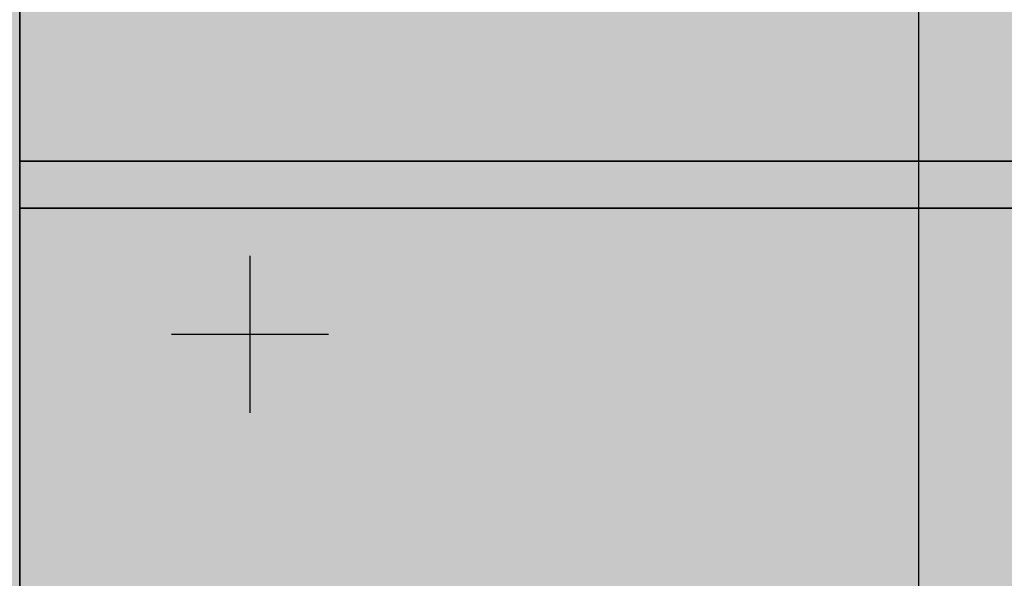
# Model space of a CAD drawing. Units: millimetres. Extents: x 130 to 1021, y 147 to 699.
# Tile 31 of 40: x 487 to 550, y 440 to 476. Entities that reach past the tile are written whole.
import ezdxf

# ---------------------------------------------------------------- set-up
doc = ezdxf.new("R2010")
doc.units = ezdxf.units.MM
doc.header["$MEASUREMENT"] = 0
for name, color, linetype, lineweight in [('A-ANNO-DIMS', 2, 'Continuous', 18), ('A-ELEV', 7, 'Continuous', 35), ('A-ELEV-PATT', 9, 'Continuous', 13)]:
    doc.layers.add(name, color=color, linetype=linetype, lineweight=lineweight)
doc.styles.get("Standard").update_dxf_attribs({"font": 'arial.ttf'})
doc.dimstyles.get("Standard").update_dxf_attribs({"dimtxt": 20, "dimasz": 10, "dimexe": 10, "dimexo": 10, "dimgap": 5, "dimtad": 0, "dimtih": 1, "dimtoh": 1, "dimdec": 0, "dimzin": 0, "dimdsep": 46, "dimtxsty": 'Standard', "dimcen": 5, "dimadec": 0, "dimazin": 0, "dimtfac": 1, "dimtdec": 0, "dimtofl": 0, "dimtmove": 0, "dimatfit": 3, "dimfxl": 1, "dimtolj": 1, "dimtzin": 0, "dimarcsym": 0})

# ---------------------------------------------------------------- blocks, each defined once
blk = doc.blocks.new('*D11')
at = {"layer": 'A-ANNO-DIMS', "color": 0, "lineweight": -2, "transparency": 16777216}
for p, q in [((737.374, 648.699), (737.374, 149.739)), ((299.374, 566.947), (299.374, 149.739)), ((309.374, 159.739), (490.857, 159.739)), ((727.374, 159.739), (545.891, 159.739))]:
    blk.add_line(p, q, dxfattribs=at)
at = {"layer": 'A-ANNO-DIMS', "color": 0, "transparency": 16777216}
for points in [[(309.374, 161.406), (309.374, 158.073), (299.374, 159.739)], [(727.374, 161.406), (727.374, 158.073), (737.374, 159.739)]]:
    blk.add_solid(points, dxfattribs=at)
at = {"layer": 'Defpoints', "color": 0, "transparency": 16777216}
for p in [(737.374, 658.699), (299.374, 576.947), (737.374, 159.739)]:
    blk.add_point(p, dxfattribs=at)
at = {"layer": 'A-ANNO-DIMS', "color": 0, "transparency": 16777216, "insert": (518.374, 159.739), "char_height": 20, "attachment_point": 5}
blk.add_mtext('\\A1;438', dxfattribs=at)
blk = doc.blocks.new('*D12')
at = {"layer": 'A-ANNO-DIMS', "color": 0, "lineweight": -2, "transparency": 16777216}
for p, q in [((477.374, 661.947), (265.074, 661.947)), ((275.074, 651.947), (275.074, 438.205)), ((275.074, 194.039), (275.074, 407.782)), ((357.163, 184.039), (265.074, 184.039))]:
    blk.add_line(p, q, dxfattribs=at)
at = {"layer": 'A-ANNO-DIMS', "color": 0, "transparency": 16777216}
for points in [[(273.407, 651.947), (276.74, 651.947), (275.074, 661.947)], [(273.407, 194.039), (276.74, 194.039), (275.074, 184.039)]]:
    blk.add_solid(points, dxfattribs=at)
at = {"layer": 'Defpoints', "color": 0, "transparency": 16777216}
for p in [(275.074, 661.947), (487.374, 661.947), (367.163, 184.039)]:
    blk.add_point(p, dxfattribs=at)
at = {"layer": 'A-ANNO-DIMS', "color": 0, "transparency": 16777216, "insert": (275.074, 422.993), "char_height": 20, "attachment_point": 5}
blk.add_mtext('\\A1;477.9', dxfattribs=at)
blk = doc.blocks.new('*D19')
at = {"layer": 'A-ANNO-DIMS', "color": 0, "lineweight": -2, "transparency": 16777216}
for p, q in [((382.374, 388.947), (382.374, 696.247)), ((414.652, 510.881), (414.652, 696.247)), ((392.374, 686.247), (404.652, 686.247)), ((414.652, 686.247), (424.652, 686.247))]:
    blk.add_line(p, q, dxfattribs=at)
at = {"layer": 'A-ANNO-DIMS', "color": 0, "transparency": 16777216}
for points in [[(392.374, 687.914), (392.374, 684.581), (382.374, 686.247)], [(404.652, 687.914), (404.652, 684.581), (414.652, 686.247)]]:
    blk.add_solid(points, dxfattribs=at)
at = {"layer": 'Defpoints', "color": 0, "transparency": 16777216}
for p in [(414.652, 686.247), (414.652, 500.881), (382.374, 378.947)]:
    blk.add_point(p, dxfattribs=at)
at = {"layer": 'A-ANNO-DIMS', "color": 0, "transparency": 16777216, "insert": (463.411, 686.247), "char_height": 20, "attachment_point": 5}
blk.add_mtext('\\A1;32.28', dxfattribs=at)
blk = doc.blocks.new('*D20')
at = {"layer": 'A-ANNO-DIMS', "color": 0, "lineweight": -2, "transparency": 16777216}
for p, q in [((414.652, 510.881), (414.652, 696.247)), ((432.374, 388.947), (432.374, 696.247)), ((404.652, 686.247), (394.652, 686.247)), ((442.374, 686.247), (452.374, 686.247))]:
    blk.add_line(p, q, dxfattribs=at)
at = {"layer": 'A-ANNO-DIMS', "color": 0, "transparency": 16777216}
for points in [[(404.652, 687.914), (404.652, 684.581), (414.652, 686.247)], [(442.374, 687.914), (442.374, 684.581), (432.374, 686.247)]]:
    blk.add_solid(points, dxfattribs=at)
at = {"layer": 'Defpoints', "color": 0, "transparency": 16777216}
for p in [(432.374, 686.247), (414.652, 500.881), (432.374, 378.947)]:
    blk.add_point(p, dxfattribs=at)
at = {"layer": 'A-ANNO-DIMS', "color": 0, "transparency": 16777216, "insert": (490.075, 686.247), "char_height": 20, "attachment_point": 5}
blk.add_mtext('\\A1;17.72', dxfattribs=at)
blk = doc.blocks.new('*D21')
at = {"layer": 'A-ANNO-DIMS', "color": 0, "lineweight": -2, "transparency": 16777216}
for p, q in [((432.374, 388.947), (432.374, 696.247)), ((447.374, 656.947), (447.374, 696.247)), ((422.374, 686.247), (412.374, 686.247)), ((457.374, 686.247), (467.374, 686.247))]:
    blk.add_line(p, q, dxfattribs=at)
at = {"layer": 'A-ANNO-DIMS', "color": 0, "transparency": 16777216}
for points in [[(422.374, 687.914), (422.374, 684.581), (432.374, 686.247)], [(457.374, 687.914), (457.374, 684.581), (447.374, 686.247)]]:
    blk.add_solid(points, dxfattribs=at)
at = {"layer": 'Defpoints', "color": 0, "transparency": 16777216}
for p in [(447.374, 686.247), (447.374, 646.947), (432.374, 378.947)]:
    blk.add_point(p, dxfattribs=at)
at = {"layer": 'A-ANNO-DIMS', "color": 0, "transparency": 16777216, "insert": (485.832, 686.247), "char_height": 20, "attachment_point": 5}
blk.add_mtext('\\A1;15', dxfattribs=at)
blk = doc.blocks.new('*D22')
at = {"layer": 'A-ANNO-DIMS', "color": 0, "lineweight": -2, "transparency": 16777216}
for p, q in [((447.374, 656.947), (447.374, 696.247)), ((466.767, 403.947), (466.767, 696.247)), ((437.374, 686.247), (427.374, 686.247)), ((476.767, 686.247), (486.767, 686.247))]:
    blk.add_line(p, q, dxfattribs=at)
at = {"layer": 'A-ANNO-DIMS', "color": 0, "transparency": 16777216}
for points in [[(437.374, 687.914), (437.374, 684.581), (447.374, 686.247)], [(476.767, 687.914), (476.767, 684.581), (466.767, 686.247)]]:
    blk.add_solid(points, dxfattribs=at)
at = {"layer": 'Defpoints', "color": 0, "transparency": 16777216}
for p in [(466.767, 686.247), (447.374, 646.947), (466.767, 393.947)]:
    blk.add_point(p, dxfattribs=at)
at = {"layer": 'A-ANNO-DIMS', "color": 0, "transparency": 16777216, "insert": (532.34, 686.247), "char_height": 20, "attachment_point": 5}
blk.add_mtext('\\A1;19.393', dxfattribs=at)
blk = doc.blocks.new('*D23')
at = {"layer": 'A-ANNO-DIMS', "color": 0, "lineweight": -2, "transparency": 16777216}
for p, q in [((466.767, 403.947), (466.767, 696.247)), ((475.988, 209.039), (475.988, 696.247)), ((456.767, 686.247), (446.767, 686.247)), ((485.988, 686.247), (495.988, 686.247))]:
    blk.add_line(p, q, dxfattribs=at)
at = {"layer": 'A-ANNO-DIMS', "color": 0, "transparency": 16777216}
for points in [[(456.767, 687.914), (456.767, 684.581), (466.767, 686.247)], [(485.988, 687.914), (485.988, 684.581), (475.988, 686.247)]]:
    blk.add_solid(points, dxfattribs=at)
at = {"layer": 'Defpoints', "color": 0, "transparency": 16777216}
for p in [(475.988, 686.247), (466.767, 393.947), (475.988, 199.039)]:
    blk.add_point(p, dxfattribs=at)
at = {"layer": 'A-ANNO-DIMS', "color": 0, "transparency": 16777216, "insert": (534.631, 686.247), "char_height": 20, "attachment_point": 5}
blk.add_mtext('\\A1;9.222', dxfattribs=at)
blk = doc.blocks.new('*D24')
at = {"layer": 'A-ANNO-DIMS', "color": 0, "lineweight": -2, "transparency": 16777216}
for p, q in [((475.988, 209.039), (475.988, 696.247)), ((487.374, 671.947), (487.374, 696.247)), ((465.988, 686.247), (455.988, 686.247)), ((497.374, 686.247), (507.374, 686.247))]:
    blk.add_line(p, q, dxfattribs=at)
at = {"layer": 'A-ANNO-DIMS', "color": 0, "transparency": 16777216}
for points in [[(465.988, 687.914), (465.988, 684.581), (475.988, 686.247)], [(497.374, 687.914), (497.374, 684.581), (487.374, 686.247)]]:
    blk.add_solid(points, dxfattribs=at)
at = {"layer": 'Defpoints', "color": 0, "transparency": 16777216}
for p in [(487.374, 686.247), (487.374, 661.947), (475.988, 199.039)]:
    blk.add_point(p, dxfattribs=at)
at = {"layer": 'A-ANNO-DIMS', "color": 0, "transparency": 16777216, "insert": (553.022, 686.247), "char_height": 20, "attachment_point": 5}
blk.add_mtext('\\A1;11.385', dxfattribs=at)
blk = doc.blocks.new('*D27')
at = {"layer": 'A-ANNO-DIMS', "color": 0, "lineweight": -2, "transparency": 16777216}
for p, q in [((502.374, 593.947), (502.374, 696.247)), ((544.635, 396.264), (544.635, 696.247)), ((512.374, 686.247), (534.635, 686.247)), ((544.635, 686.247), (554.635, 686.247))]:
    blk.add_line(p, q, dxfattribs=at)
at = {"layer": 'A-ANNO-DIMS', "color": 0, "transparency": 16777216}
for points in [[(512.374, 687.914), (512.374, 684.581), (502.374, 686.247)], [(534.635, 687.914), (534.635, 684.581), (544.635, 686.247)]]:
    blk.add_solid(points, dxfattribs=at)
at = {"layer": 'Defpoints', "color": 0, "transparency": 16777216}
for p in [(544.635, 686.247), (502.374, 583.947), (544.635, 386.264)]:
    blk.add_point(p, dxfattribs=at)
at = {"layer": 'A-ANNO-DIMS', "color": 0, "transparency": 16777216, "insert": (593.776, 686.247), "char_height": 20, "attachment_point": 5}
blk.add_mtext('\\A1;42.26', dxfattribs=at)
blk = doc.blocks.new('*D28')
at = {"layer": 'A-ANNO-DIMS', "color": 0, "lineweight": -2, "transparency": 16777216}
for p, q in [((544.635, 396.264), (544.635, 696.247)), ((552.374, 593.947), (552.374, 696.247)), ((534.635, 686.247), (524.635, 686.247)), ((562.374, 686.247), (572.374, 686.247))]:
    blk.add_line(p, q, dxfattribs=at)
at = {"layer": 'A-ANNO-DIMS', "color": 0, "transparency": 16777216}
for points in [[(534.635, 687.914), (534.635, 684.581), (544.635, 686.247)], [(562.374, 687.914), (562.374, 684.581), (552.374, 686.247)]]:
    blk.add_solid(points, dxfattribs=at)
at = {"layer": 'Defpoints', "color": 0, "transparency": 16777216}
for p in [(552.374, 686.247), (552.374, 583.947), (544.635, 386.264)]:
    blk.add_point(p, dxfattribs=at)
at = {"layer": 'A-ANNO-DIMS', "color": 0, "transparency": 16777216, "insert": (611.057, 686.247), "char_height": 20, "attachment_point": 5}
blk.add_mtext('\\A1;7.738', dxfattribs=at)
blk = doc.blocks.new('*D54')
at = {"layer": 'A-ANNO-DIMS', "color": 0, "lineweight": -2, "transparency": 16777216}
for p, q in [((761.674, 473.947), (761.674, 483.947)), ((497.374, 463.947), (771.674, 463.947)), ((747.374, 403.69), (771.674, 403.69)), ((761.674, 393.69), (761.674, 383.69))]:
    blk.add_line(p, q, dxfattribs=at)
at = {"layer": 'A-ANNO-DIMS', "color": 0, "transparency": 16777216}
for points in [[(760.007, 473.947), (763.34, 473.947), (761.674, 463.947)], [(760.007, 393.69), (763.34, 393.69), (761.674, 403.69)]]:
    blk.add_solid(points, dxfattribs=at)
at = {"layer": 'Defpoints', "color": 0, "transparency": 16777216}
for p in [(487.374, 463.947), (761.674, 463.947), (737.374, 403.69)]:
    blk.add_point(p, dxfattribs=at)
at = {"layer": 'A-ANNO-DIMS', "color": 0, "transparency": 16777216, "insert": (761.674, 433.819), "char_height": 20, "attachment_point": 5}
blk.add_mtext('\\A1;60.26', dxfattribs=at)
blk = doc.blocks.new('*D55')
at = {"layer": 'A-ANNO-DIMS', "color": 0, "lineweight": -2, "transparency": 16777216}
for p, q in [((761.674, 486.947), (761.674, 496.947)), ((761.674, 496.947), (771.674, 496.947)), ((562.374, 476.947), (771.674, 476.947)), ((497.374, 463.947), (771.674, 463.947)), ((761.674, 453.947), (761.674, 443.947))]:
    blk.add_line(p, q, dxfattribs=at)
at = {"layer": 'A-ANNO-DIMS', "color": 0, "transparency": 16777216}
for points in [[(760.007, 486.947), (763.34, 486.947), (761.674, 476.947)], [(760.007, 453.947), (763.34, 453.947), (761.674, 463.947)]]:
    blk.add_solid(points, dxfattribs=at)
at = {"layer": 'Defpoints', "color": 0, "transparency": 16777216}
for p in [(552.374, 476.947), (761.674, 476.947), (487.374, 463.947)]:
    blk.add_point(p, dxfattribs=at)
at = {"layer": 'A-ANNO-DIMS', "color": 0, "transparency": 16777216, "insert": (790.057, 496.947), "char_height": 20, "attachment_point": 5}
blk.add_mtext('\\A1;13', dxfattribs=at)
blk = doc.blocks.new('*D64')
at = {"layer": 'A-ANNO-DIMS', "color": 0, "lineweight": -2, "transparency": 16777216}
for p, q in [((502.049, 450.926), (502.049, 460.926)), ((497.049, 455.926), (507.049, 455.926)), ((363.96, 263.061), (409.922, 327.255)), ((353.96, 263.061), (363.96, 263.061))]:
    blk.add_line(p, q, dxfattribs=at)
at = {"layer": 'A-ANNO-DIMS', "color": 0, "transparency": 16777216}
blk.add_solid([(408.567, 328.225), (411.277, 326.284), (415.743, 335.385)], dxfattribs=at)
at = {"layer": 'Defpoints', "color": 0, "transparency": 16777216}
for p in [(502.049, 455.926), (415.743, 335.385)]:
    blk.add_point(p, dxfattribs=at)
at = {"layer": 'A-ANNO-DIMS', "color": 0, "transparency": 16777216, "insert": (297.8, 263.061), "char_height": 20, "attachment_point": 5}
blk.add_mtext('\\A1;R148.25', dxfattribs=at)
blk = doc.blocks.new('*D65')
at = {"layer": 'A-ANNO-DIMS', "color": 0, "lineweight": -2, "transparency": 16777216}
for p, q in [((495.463, 509.127), (472.508, 423.108)), ((505.463, 509.127), (495.463, 509.127)), ((427.374, 248.979), (427.374, 258.979)), ((422.374, 253.979), (432.374, 253.979))]:
    blk.add_line(p, q, dxfattribs=at)
at = {"layer": 'A-ANNO-DIMS', "color": 0, "transparency": 16777216}
blk.add_solid([(470.898, 423.538), (474.118, 422.679), (469.93, 413.447)], dxfattribs=at)
at = {"layer": 'Defpoints', "color": 0, "transparency": 16777216}
for p in [(469.93, 413.447), (427.374, 253.979)]:
    blk.add_point(p, dxfattribs=at)
at = {"layer": 'A-ANNO-DIMS', "color": 0, "transparency": 16777216, "insert": (561.623, 509.127), "char_height": 20, "attachment_point": 5}
blk.add_mtext('\\A1;R165.05', dxfattribs=at)
blk = doc.blocks.new('*D67')
at = {"layer": 'A-ANNO-DIMS', "color": 0, "lineweight": -2, "transparency": 16777216}
for p, q in [((479.756, 492.431), (462.144, 412.223)), ((489.756, 492.431), (479.756, 492.431)), ((427.07, 247.496), (427.07, 257.496)), ((422.07, 252.496), (432.07, 252.496))]:
    blk.add_line(p, q, dxfattribs=at)
at = {"layer": 'A-ANNO-DIMS', "color": 0, "transparency": 16777216}
blk.add_solid([(460.516, 412.58), (463.772, 411.865), (459.999, 402.455)], dxfattribs=at)
at = {"layer": 'Defpoints', "color": 0, "transparency": 16777216}
for p in [(459.999, 402.455), (427.07, 252.496)]:
    blk.add_point(p, dxfattribs=at)
at = {"layer": 'A-ANNO-DIMS', "color": 0, "transparency": 16777216, "insert": (545.841, 492.431), "char_height": 20, "attachment_point": 5}
blk.add_mtext('\\A1;R153.53', dxfattribs=at)
blk = doc.blocks.new('*D69')
at = {"layer": 'A-ANNO-DIMS', "color": 0, "lineweight": -2, "transparency": 16777216}
for p, q in [((507.746, 572.261), (483.091, 501.813)), ((517.746, 572.261), (507.746, 572.261)), ((433.191, 354.23), (433.191, 364.23)), ((428.191, 359.23), (438.191, 359.23))]:
    blk.add_line(p, q, dxfattribs=at)
at = {"layer": 'A-ANNO-DIMS', "color": 0, "transparency": 16777216}
blk.add_solid([(481.518, 502.363), (484.664, 501.262), (479.788, 492.374)], dxfattribs=at)
at = {"layer": 'Defpoints', "color": 0, "transparency": 16777216}
for p in [(479.788, 492.374), (433.191, 359.23)]:
    blk.add_point(p, dxfattribs=at)
at = {"layer": 'A-ANNO-DIMS', "color": 0, "transparency": 16777216, "insert": (573.824, 572.261), "char_height": 20, "attachment_point": 5}
blk.add_mtext('\\A1;R141.06', dxfattribs=at)
blk = doc.blocks.new('*D71')
at = {"layer": 'A-ANNO-DIMS', "color": 0, "lineweight": -2, "transparency": 16777216}
for p, q in [((492.108, 581.609), (472.542, 512.666)), ((502.108, 581.609), (492.108, 581.609)), ((432.65, 367.109), (432.65, 377.109)), ((427.65, 372.109), (437.65, 372.109))]:
    blk.add_line(p, q, dxfattribs=at)
at = {"layer": 'A-ANNO-DIMS', "color": 0, "transparency": 16777216}
blk.add_solid([(470.938, 513.121), (474.145, 512.211), (469.812, 503.046)], dxfattribs=at)
at = {"layer": 'Defpoints', "color": 0, "transparency": 16777216}
for p in [(469.812, 503.046), (432.65, 372.109)]:
    blk.add_point(p, dxfattribs=at)
at = {"layer": 'A-ANNO-DIMS', "color": 0, "transparency": 16777216, "insert": (548.493, 581.609), "char_height": 20, "attachment_point": 5}
blk.add_mtext('\\A1;R136.1', dxfattribs=at)
blk = doc.blocks.new('*D72')
at = {"layer": 'A-ANNO-DIMS', "color": 0, "lineweight": -2, "transparency": 16777216}
for p, q in [((460.658, 573.64), (451.279, 503.49)), ((470.658, 573.64), (460.658, 573.64)), ((432.115, 355.142), (432.115, 365.142)), ((427.115, 360.142), (437.115, 360.142))]:
    blk.add_line(p, q, dxfattribs=at)
at = {"layer": 'A-ANNO-DIMS', "color": 0, "transparency": 16777216}
blk.add_solid([(449.628, 503.711), (452.931, 503.27), (449.954, 493.579)], dxfattribs=at)
at = {"layer": 'Defpoints', "color": 0, "transparency": 16777216}
for p in [(449.954, 493.579), (432.115, 360.142)]:
    blk.add_point(p, dxfattribs=at)
at = {"layer": 'A-ANNO-DIMS', "color": 0, "transparency": 16777216, "insert": (526.64, 573.64), "char_height": 20, "attachment_point": 5}
blk.add_mtext('\\A1;R134.62', dxfattribs=at)

msp = doc.modelspace()

# ---------------------------------------------------------------- hatches: boundary and pattern name
at = {"layer": 'A-ELEV-PATT'}
h = msp.add_hatch(color=256, dxfattribs=at)
h.dxf.hatch_style = 1
h.paths.add_polyline_path([(737.3738, 658.6988, 0.0135961), (632.4019, 661.9473), (607.3738, 661.9473), (487.3738, 661.9473), (487.3738, 649.9473), (607.3738, 649.9473), (632.3794, 649.9473, -0.0136841), (737.3738, 646.6784)])
h.paths.add_polyline_path([(732.3738, 643.9599, 0.0130529), (632.3738, 646.9473), (607.3738, 646.9473), (487.3738, 646.9473), (487.3738, 596.9473), (632.3738, 596.9473, -0.0130529), (732.3738, 593.9599)])
h.paths.add_polyline_path([(737.3738, 593.6732, 0.0137063), (632.3738, 596.9473), (487.3738, 596.9473), (487.3738, 586.9473), (632.355, 586.9473, -0.0137808), (737.3738, 583.6559)])
h.paths.add_polyline_path([(447.3738, 646.9473), (307.3738, 646.9473), (302.3738, 646.9473), (302.3738, 634.9473), (447.3738, 634.9473)])
h.paths.add_polyline_path([(447.3738, 631.9473), (307.3738, 631.9473), (307.3738, 586.9473), (447.3738, 586.9473)])
h.paths.add_polyline_path([(447.3738, 586.9473), (307.3738, 586.9473), (302.3738, 586.9473), (302.3738, 576.9473), (447.3738, 576.9473)])
h.paths.add_polyline_path([(447.3738, 573.9473), (367.3738, 573.9473), (367.3738, 539.9473), (447.3738, 539.9473)])
h.paths.add_polyline_path([(447.3738, 537.9473), (367.3738, 537.9473), (367.3738, 507.9473), (400.392, 507.4253, -0.001728), (401.3281, 507.6451, -0.5220025), (425.6117, 511.0391, -0.0391849), (447.3738, 510.4359), (447.3738, 510.7883)])
h.paths.add_polyline_path([(394.7238, 505.9473), (367.3738, 505.9473), (367.3738, 476.9473, -0.0146512), (375.8501, 480.2159), (376.1506, 499.2266, -0.0355419)])
h.paths.add_polyline_path([(632.3738, 583.9473), (552.3738, 583.9473), (552.3738, 550.9473), (632.3738, 550.9473)])
h.paths.add_polyline_path([(632.3738, 548.9473), (552.3738, 548.9473), (552.3738, 515.9473), (632.3738, 515.9473)])
h.paths.add_polyline_path([(632.3738, 513.9473), (552.3738, 513.9473), (552.3738, 476.9473), (632.3738, 476.9473)])
h.paths.add_polyline_path([(737.3738, 473.6903, 0.0136326), (632.3926, 476.9473), (552.3738, 476.9473), (487.3738, 476.9473), (487.3738, 466.9473), (632.3738, 466.9473, -0.0137063), (737.3738, 463.6732)])
h.paths.add_polyline_path([(732.3738, 460.9552, 0.0130741), (632.3681, 463.9473), (487.3738, 463.9473), (487.3738, 407.735, -0.0032286), (489.3544, 406.9473), (632.3926, 406.9473, -0.0129826), (732.3738, 403.9755)])
h.paths.add_polyline_path([(487.3738, 463.9473, 0.20133), (367.3738, 463.9473), (367.3738, 407.735, -0.1882031), (487.3738, 407.735)])
h.paths.add_polyline_path([(367.3738, 476.9473), (367.3738, 466.9473, -0.2013309), (487.3738, 466.9473), (487.3738, 476.9473, 0.20133)])
h.paths.add_polyline_path([(367.3738, 463.9473), (307.3738, 463.9473), (307.3738, 401.9473), (357.9413, 401.9473), (367.3738, 407.735)])
h.paths.add_polyline_path([(367.3738, 476.9473), (302.3738, 476.9473), (302.3738, 466.9473), (367.3738, 466.9473)])
h.paths.add_polyline_path([(632.8184, 366.9453), (552.3738, 366.9453), (552.3738, 393.9473), (632.8184, 393.9473)])
h.paths.add_polyline_path([(632.8184, 357.2114), (632.8184, 363.9453), (552.3738, 363.9453), (552.3738, 357.2114), (552.3738, 336.9453), (632.8184, 336.9453)])
h.paths.add_polyline_path([(632.8184, 333.9453), (552.3738, 333.9453), (552.3738, 306.9453), (632.8184, 306.9453)])
h.paths.add_polyline_path([(632.8184, 303.9453), (552.3738, 303.9453), (552.3738, 273.9473), (632.355, 273.9473, 0.0000608), (632.8184, 273.9491)])
h.paths.add_polyline_path([(737.3738, 403.6903, 0.0136326), (632.3926, 406.9473), (489.3544, 406.9473, 0.1915481), (367.3738, 407.735), (367.3738, 396.9473, -0.2013309), (487.3738, 396.9473), (632.3738, 396.9473, -0.0137063), (737.3738, 393.6732)])
h.paths.add_polyline_path([(357.9413, 401.9473), (307.3738, 401.9473), (307.3738, 391.9473), (357.9413, 391.9473)])
h.paths.add_polyline_path([(357.9413, 357.2114), (357.9413, 388.9473), (307.3738, 388.9473), (307.3738, 357.2114), (307.3738, 273.9473), (357.9413, 273.9473)])
h.paths.add_polyline_path([(732.3738, 263.93, -0.0130317), (632.3794, 260.9473), (466.7667, 260.9473), (466.7667, 240.9473), (469.8406, 236.978), (469.8406, 221.978), (472.9145, 218.0087), (472.9145, 213.9473), (607.3738, 213.9473), (732.3738, 213.9473)])
h.paths.add_polyline_path([(732.3738, 290.889), (722.479, 290.889), (722.479, 301.889), (732.3738, 301.889), (732.3738, 305.889), (722.479, 305.889), (722.479, 316.889), (732.3738, 316.889), (732.3738, 320.889), (722.479, 320.889), (722.479, 331.889), (732.3738, 331.889), (732.3738, 335.889), (722.479, 335.889), (722.479, 346.889), (732.3738, 346.889), (732.3738, 350.889), (722.479, 350.889), (722.479, 361.889), (732.3738, 361.889), (732.3738, 365.889), (722.479, 365.889), (722.479, 376.889), (732.3738, 376.889), (732.3738, 380.889), (722.479, 380.889), (722.479, 391.4848, 0.0005233), (718.479, 391.6843), (718.479, 380.889), (707.479, 380.889), (707.479, 392.1896, 0.0005231), (703.479, 392.3576), (703.479, 380.889), (692.479, 380.889), (692.479, 392.7765, 0.0005229), (688.479, 392.9131), (688.479, 380.889), (677.479, 380.889), (677.479, 393.2456, 0.0005228), (673.479, 393.3508), (673.479, 380.889), (662.479, 380.889), (662.479, 393.597, 0.0005227), (658.479, 393.6709), (658.479, 380.889), (647.479, 380.889), (647.479, 393.8308, 0.0005226), (643.479, 393.8732), (643.479, 380.889), (632.8184, 380.889), (632.8184, 376.889), (643.479, 376.889), (643.479, 365.889), (632.8184, 365.889), (632.8184, 361.889), (643.479, 361.889), (643.479, 350.889), (632.8184, 350.889), (632.8184, 346.889), (643.479, 346.889), (643.479, 335.889), (632.8184, 335.889), (632.8184, 331.889), (643.479, 331.889), (643.479, 320.889), (632.8184, 320.889), (632.8184, 316.889), (643.479, 316.889), (643.479, 305.889), (632.8184, 305.889), (632.8184, 301.889), (643.479, 301.889), (643.479, 290.889), (632.8184, 290.889), (632.8184, 286.889), (643.479, 286.889), (643.479, 274.0217, 0.0005246), (647.479, 274.0643), (647.479, 286.889), (658.479, 286.889), (658.479, 274.2248, 0.0005246), (662.479, 274.2989), (662.479, 286.889), (673.479, 286.889), (673.479, 274.546, 0.0005247), (677.479, 274.6516), (677.479, 286.889), (688.479, 286.889), (688.479, 274.9853, 0.0005248), (692.479, 275.1224), (692.479, 286.889), (703.479, 286.889), (703.479, 275.5429, 0.000525), (707.479, 275.7115), (707.479, 286.889), (718.479, 286.889), (718.479, 276.2187, 0.0005252), (722.479, 276.4189), (722.479, 286.889), (732.3738, 286.889)])
h.paths.add_polyline_path([(718.479, 290.889), (707.479, 290.889), (707.479, 301.889), (718.479, 301.889)], flags=16)
h.paths.add_polyline_path([(703.479, 290.889), (692.479, 290.889), (692.479, 301.889), (703.479, 301.889)], flags=16)
h.paths.add_polyline_path([(718.479, 305.889), (707.479, 305.889), (707.479, 316.889), (718.479, 316.889)], flags=16)
h.paths.add_polyline_path([(703.479, 305.889), (692.479, 305.889), (692.479, 316.889), (703.479, 316.889)], flags=16)
h.paths.add_polyline_path([(688.479, 290.889), (677.479, 290.889), (677.479, 301.889), (688.479, 301.889)], flags=16)
h.paths.add_polyline_path([(718.479, 320.889), (707.479, 320.889), (707.479, 331.889), (718.479, 331.889)], flags=16)
h.paths.add_polyline_path([(688.479, 305.889), (677.479, 305.889), (677.479, 316.889), (688.479, 316.889)], flags=16)
h.paths.add_polyline_path([(703.479, 320.889), (692.479, 320.889), (692.479, 331.889), (703.479, 331.889)], flags=16)
h.paths.add_polyline_path([(688.479, 320.889), (677.479, 320.889), (677.479, 331.889), (688.479, 331.889)], flags=16)
h.paths.add_polyline_path([(673.479, 290.889), (662.479, 290.889), (662.479, 301.889), (673.479, 301.889)], flags=16)
h.paths.add_polyline_path([(718.479, 335.889), (707.479, 335.889), (707.479, 346.889), (718.479, 346.889)], flags=16)
h.paths.add_polyline_path([(673.479, 305.889), (662.479, 305.889), (662.479, 316.889), (673.479, 316.889)], flags=16)
h.paths.add_polyline_path([(703.479, 335.889), (692.479, 335.889), (692.479, 346.889), (703.479, 346.889)], flags=16)
h.paths.add_polyline_path([(673.479, 320.889), (662.479, 320.889), (662.479, 331.889), (673.479, 331.889)], flags=16)
h.paths.add_polyline_path([(688.479, 335.889), (677.479, 335.889), (677.479, 346.889), (688.479, 346.889)], flags=16)
h.paths.add_polyline_path([(658.479, 290.889), (647.479, 290.889), (647.479, 301.889), (658.479, 301.889)], flags=16)
h.paths.add_polyline_path([(718.479, 350.889), (707.479, 350.889), (707.479, 361.889), (718.479, 361.889)], flags=16)
h.paths.add_polyline_path([(658.479, 305.889), (647.479, 305.889), (647.479, 316.889), (658.479, 316.889)], flags=16)
h.paths.add_polyline_path([(703.479, 350.889), (692.479, 350.889), (692.479, 361.889), (703.479, 361.889)], flags=16)
h.paths.add_polyline_path([(673.479, 335.889), (662.479, 335.889), (662.479, 346.889), (673.479, 346.889)], flags=16)
h.paths.add_polyline_path([(658.479, 320.889), (647.479, 320.889), (647.479, 331.889), (658.479, 331.889)], flags=16)
h.paths.add_polyline_path([(688.479, 350.889), (677.479, 350.889), (677.479, 361.889), (688.479, 361.889)], flags=16)
h.paths.add_polyline_path([(718.479, 365.889), (707.479, 365.889), (707.479, 376.889), (718.479, 376.889)], flags=16)
h.paths.add_polyline_path([(658.479, 335.889), (647.479, 335.889), (647.479, 346.889), (658.479, 346.889)], flags=16)
h.paths.add_polyline_path([(673.479, 350.889), (662.479, 350.889), (662.479, 361.889), (673.479, 361.889)], flags=16)
h.paths.add_polyline_path([(703.479, 365.889), (692.479, 365.889), (692.479, 376.889), (703.479, 376.889)], flags=16)
h.paths.add_polyline_path([(688.479, 365.889), (677.479, 365.889), (677.479, 376.889), (688.479, 376.889)], flags=16)
h.paths.add_polyline_path([(658.479, 350.889), (647.479, 350.889), (647.479, 361.889), (658.479, 361.889)], flags=16)
h.paths.add_polyline_path([(673.479, 365.889), (662.479, 365.889), (662.479, 376.889), (673.479, 376.889)], flags=16)
h.paths.add_polyline_path([(658.479, 365.889), (647.479, 365.889), (647.479, 376.889), (658.479, 376.889)], flags=16)
h.paths.add_polyline_path([(732.3738, 503.9786), (722.3392, 503.9786), (722.3392, 514.9786), (732.3738, 514.9786), (732.3738, 518.9786), (722.3392, 518.9786), (722.3392, 529.9786), (732.3738, 529.9786), (732.3738, 533.9786), (722.3392, 533.9786), (722.3392, 544.9786), (732.3738, 544.9786), (732.3738, 546.9473), (732.3738, 548.9786), (722.3392, 548.9786), (722.3392, 559.9786), (732.3738, 559.9786), (732.3738, 563.9786), (722.3392, 563.9786), (722.3392, 574.9786), (732.3738, 574.9786), (732.3738, 578.9786), (722.3392, 578.9786), (722.3392, 581.4789, 0.000526), (718.3392, 581.6791), (718.3392, 578.9786), (707.3392, 578.9786), (707.3392, 582.1863, 0.0005258), (703.3392, 582.355), (703.3392, 578.9786), (692.3392, 578.9786), (692.3392, 582.7752, 0.0005257), (688.3392, 582.9123), (688.3392, 578.9786), (677.3392, 578.9786), (677.3392, 583.2457, 0.0005255), (673.3392, 583.3512), (673.3392, 578.9786), (662.3392, 578.9786), (662.3392, 583.5978, 0.0005254), (658.3392, 583.6718), (658.3392, 578.9786), (647.3392, 578.9786), (647.3392, 583.8317, 0.0005254), (643.3392, 583.8741), (643.3392, 578.9786), (632.3738, 578.9786), (632.3738, 574.9786), (643.3392, 574.9786), (643.3392, 563.9786), (632.3738, 563.9786), (632.3738, 559.9786), (643.3392, 559.9786), (643.3392, 548.9786), (632.3738, 548.9786), (632.3738, 544.9786), (643.3392, 544.9786), (643.3392, 533.9786), (632.3738, 533.9786), (632.3738, 529.9786), (643.3392, 529.9786), (643.3392, 518.9786), (632.3738, 518.9786), (632.3738, 515.9473), (632.3738, 514.9786), (643.3392, 514.9786), (643.3392, 503.9786), (632.3738, 503.9786), (632.3738, 499.9786), (643.3392, 499.9786), (643.3392, 488.9786), (632.3738, 488.9786), (632.3738, 484.9786), (643.3392, 484.9786), (643.3392, 476.8751, -0.0005191), (647.3392, 476.8332), (647.3392, 484.9786), (658.3392, 484.9786), (658.3392, 476.6752, -0.0005192), (662.3392, 476.6022), (662.3392, 484.9786), (673.3392, 484.9786), (673.3392, 476.3585, -0.0005193), (677.3392, 476.2543), (677.3392, 484.9786), (688.3392, 484.9786), (688.3392, 475.9248, -0.0005194), (692.3392, 475.7894), (692.3392, 484.9786), (703.3392, 484.9786), (703.3392, 475.3741, -0.0005195), (707.3392, 475.2075), (707.3392, 484.9786), (718.3392, 484.9786), (718.3392, 474.7064, -0.0005197), (722.3392, 474.5086), (722.3392, 484.9786), (732.3738, 484.9786), (732.3738, 488.9786), (722.3392, 488.9786), (722.3392, 499.9786), (732.3738, 499.9786)])
h.paths.add_polyline_path([(718.3392, 503.9786), (707.3392, 503.9786), (707.3392, 514.9786), (718.3392, 514.9786)], flags=16)
h.paths.add_polyline_path([(718.3392, 499.9786), (718.3392, 488.9786), (707.3392, 488.9786), (707.3392, 499.9786)], flags=16)
h.paths.add_polyline_path([(718.3392, 518.9786), (707.3392, 518.9786), (707.3392, 529.9786), (718.3392, 529.9786)], flags=16)
h.paths.add_polyline_path([(703.3392, 503.9786), (692.3392, 503.9786), (692.3392, 514.9786), (703.3392, 514.9786)], flags=16)
h.paths.add_polyline_path([(703.3392, 499.9786), (703.3392, 488.9786), (692.3392, 488.9786), (692.3392, 499.9786)], flags=16)
h.paths.add_polyline_path([(703.3392, 518.9786), (692.3392, 518.9786), (692.3392, 529.9786), (703.3392, 529.9786)], flags=16)
h.paths.add_polyline_path([(718.3392, 533.9786), (707.3392, 533.9786), (707.3392, 544.9786), (718.3392, 544.9786)], flags=16)
h.paths.add_polyline_path([(688.3392, 503.9786), (677.3392, 503.9786), (677.3392, 514.9786), (688.3392, 514.9786)], flags=16)
h.paths.add_polyline_path([(688.3392, 499.9786), (688.3392, 488.9786), (677.3392, 488.9786), (677.3392, 499.9786)], flags=16)
h.paths.add_polyline_path([(703.3392, 533.9786), (692.3392, 533.9786), (692.3392, 544.9786), (703.3392, 544.9786)], flags=16)
h.paths.add_polyline_path([(688.3392, 518.9786), (677.3392, 518.9786), (677.3392, 529.9786), (688.3392, 529.9786)], flags=16)
h.paths.add_polyline_path([(688.3392, 533.9786), (677.3392, 533.9786), (677.3392, 544.9786), (688.3392, 544.9786)], flags=16)
h.paths.add_polyline_path([(718.3392, 548.9786), (707.3392, 548.9786), (707.3392, 559.9786), (718.3392, 559.9786)], flags=16)
h.paths.add_polyline_path([(673.3392, 503.9786), (662.3392, 503.9786), (662.3392, 514.9786), (673.3392, 514.9786)], flags=16)
h.paths.add_polyline_path([(673.3392, 499.9786), (673.3392, 488.9786), (662.3392, 488.9786), (662.3392, 499.9786)], flags=16)
h.paths.add_polyline_path([(703.3392, 548.9786), (692.3392, 548.9786), (692.3392, 559.9786), (703.3392, 559.9786)], flags=16)
h.paths.add_polyline_path([(673.3392, 518.9786), (662.3392, 518.9786), (662.3392, 529.9786), (673.3392, 529.9786)], flags=16)
h.paths.add_polyline_path([(688.3392, 548.9786), (677.3392, 548.9786), (677.3392, 559.9786), (688.3392, 559.9786)], flags=16)
h.paths.add_polyline_path([(673.3392, 533.9786), (662.3392, 533.9786), (662.3392, 544.9786), (673.3392, 544.9786)], flags=16)
h.paths.add_polyline_path([(718.3392, 563.9786), (707.3392, 563.9786), (707.3392, 574.9786), (718.3392, 574.9786)], flags=16)
h.paths.add_polyline_path([(658.3392, 503.9786), (647.3392, 503.9786), (647.3392, 514.9786), (658.3392, 514.9786)], flags=16)
h.paths.add_polyline_path([(658.3392, 499.9786), (658.3392, 488.9786), (647.3392, 488.9786), (647.3392, 499.9786)], flags=16)
h.paths.add_polyline_path([(703.3392, 563.9786), (692.3392, 563.9786), (692.3392, 574.9786), (703.3392, 574.9786)], flags=16)
h.paths.add_polyline_path([(658.3392, 518.9786), (647.3392, 518.9786), (647.3392, 529.9786), (658.3392, 529.9786)], flags=16)
h.paths.add_polyline_path([(673.3392, 548.9786), (662.3392, 548.9786), (662.3392, 559.9786), (673.3392, 559.9786)], flags=16)
h.paths.add_polyline_path([(688.3392, 563.9786), (677.3392, 563.9786), (677.3392, 574.9786), (688.3392, 574.9786)], flags=16)
h.paths.add_polyline_path([(658.3392, 533.9786), (647.3392, 533.9786), (647.3392, 544.9786), (658.3392, 544.9786)], flags=16)
h.paths.add_polyline_path([(673.3392, 563.9786), (662.3392, 563.9786), (662.3392, 574.9786), (673.3392, 574.9786)], flags=16)
h.paths.add_polyline_path([(658.3392, 548.9786), (647.3392, 548.9786), (647.3392, 559.9786), (658.3392, 559.9786)], flags=16)
h.paths.add_polyline_path([(658.3392, 563.9786), (647.3392, 563.9786), (647.3392, 574.9786), (658.3392, 574.9786)], flags=16)
h = msp.add_hatch(color=256, dxfattribs=at)
h.dxf.hatch_style = 1
h.paths.add_polyline_path([(447.3738, 576.9473), (302.3738, 576.9473), (302.3738, 573.9473), (447.3738, 573.9473)])
h.paths.add_polyline_path([(487.3738, 583.9473), (487.3738, 586.9473), (447.3738, 576.9473), (447.3738, 573.9473)])
h.paths.add_polyline_path([(632.355, 586.9473), (487.3738, 586.9473), (487.3738, 583.9473), (632.3738, 583.9473), (632.3738, 583.9472, -0.0138), (737.3738, 580.6507), (737.3738, 583.6559, 0.0137808)])
h.paths.add_polyline_path([(367.3738, 466.9473), (302.3738, 466.9473), (302.3738, 463.9473), (367.3738, 463.9473)])
h.paths.add_polyline_path([(487.3738, 463.9473), (487.3738, 466.9473, 0.2013309), (367.3738, 466.9473), (367.3738, 463.9473, -0.20133)])
h.paths.add_polyline_path([(632.3738, 466.9473), (487.3738, 466.9473), (487.3738, 463.9473), (632.3681, 463.9473, -0.0137285), (737.3738, 460.6681), (737.3738, 463.6732, 0.0137063)])
h.paths.add_polyline_path([(632.3738, 396.9473), (487.3738, 396.9473, 0.2013309), (367.3738, 396.9473), (367.3738, 393.9473, -0.2023717), (486.7667, 393.9473), (632.3681, 393.9473, -0.0137285), (737.3738, 390.6681), (737.3738, 393.6732, 0.0137063)])
h.paths.add_polyline_path([(357.9413, 391.9473), (307.3738, 391.9473), (307.3738, 388.9473), (357.9413, 388.9473)])
h.paths.add_polyline_path([(367.3738, 393.9473), (367.3738, 396.9473), (357.9413, 391.924), (357.9413, 388.9473), (358.058, 388.9473)])
h.paths.add_polyline_path([(737.3738, 264.2162), (737.3738, 267.2214, -0.0137063), (632.3738, 263.9473), (463.7667, 263.9473), (466.7667, 260.9473), (632.3794, 260.9473, 0.0136841)])
h.paths.add_polyline_path([(463.7667, 263.9473), (447.3738, 263.9473), (450.3738, 260.9473), (466.7667, 260.9473)])
h.paths.add_polyline_path([(447.3738, 263.9473), (432.3738, 263.9473), (432.3738, 260.9473), (450.3738, 260.9473)])
h.paths.add_polyline_path([(382.3738, 263.9473), (357.9413, 263.9473), (357.9413, 260.9473), (382.3738, 260.9473)])
h.paths.add_polyline_path([(357.9413, 263.9473), (307.3738, 263.9473), (307.3738, 260.9473), (357.9413, 260.9473)])

# ---------------------------------------------------------------- linework, layer by layer
at = {"layer": 'A-ELEV'}
for p, q in [((487.3738, 407.735), (487.3738, 476.9473)), ((632.3738, 466.9473), (487.3738, 466.9473)), ((632.3738, 463.9473), (487.3738, 463.9473))]:
    msp.add_line(p, q, dxfattribs=at)

# ---------------------------------------------------------------- dimensions: what is measured, and where the dimension line sits
at = {"layer": 'A-ANNO-DIMS'}
for base, p1, p2, override, picture, middle in [((414.6525, 686.2473), (382.3738, 378.9473), (414.6525, 500.8811), {"dimdec": 2, "dimlfac": 1, "dimrnd": 0, "dimzin": 0, "dimdsep": 46, "dimlunit": 2}, '*D19', (463.411, 686.2473)), ((432.3738, 686.2473), (414.6525, 500.8811), (432.3738, 378.9473), {"dimdec": 2, "dimlfac": 1, "dimrnd": 0, "dimzin": 0, "dimdsep": 46, "dimlunit": 2}, '*D20', (490.075, 686.2473)), ((447.3738, 686.2473), (432.3738, 378.9473), (447.3738, 646.9473), {"dimdec": 0, "dimlfac": 1, "dimrnd": 0, "dimzin": 0, "dimdsep": 46, "dimlunit": 2}, '*D21', (485.8322, 686.2473)), ((466.7667, 686.2473), (447.3738, 646.9473), (466.7667, 393.9473), {"dimdec": 3, "dimlfac": 1, "dimrnd": 0, "dimzin": 0, "dimdsep": 46, "dimlunit": 2}, '*D22', (532.3397, 686.2473)), ((475.9885, 686.2473), (466.7667, 393.9473), (475.9885, 199.0395), {"dimdec": 3, "dimlfac": 1, "dimrnd": 0, "dimzin": 0, "dimdsep": 46, "dimlunit": 2}, '*D23', (534.631, 686.2473)), ((487.3738, 686.2473), (475.9885, 199.0395), (487.3738, 661.9473), {"dimdec": 3, "dimlfac": 1, "dimrnd": 0, "dimzin": 0, "dimdsep": 46, "dimlunit": 2}, '*D24', (553.0218, 686.2473)), ((544.6354, 686.2473), (502.3738, 583.9473), (544.6354, 386.2639), {"dimdec": 2, "dimlfac": 1, "dimrnd": 0, "dimzin": 0, "dimdsep": 46, "dimlunit": 2}, '*D27', (593.776, 686.2473)), ((552.3738, 686.2473), (544.6354, 386.2639), (552.3738, 583.9473), {"dimdec": 3, "dimlfac": 1, "dimrnd": 0, "dimzin": 0, "dimdsep": 46, "dimlunit": 2}, '*D28', (611.0573, 686.2473)), ((737.3738, 159.7395), (299.3738, 576.9473), (737.3738, 658.6988), {"dimdec": 0, "dimlfac": 1, "dimrnd": 0, "dimzin": 0, "dimdsep": 46, "dimlunit": 2}, '*D11', (518.3738, 159.7395))]:
    dim = msp.add_linear_dim(base=base, p1=p1, p2=p2, dimstyle='Standard', override=override, dxfattribs=at)
    dim.commit()
    dim.dimension.update_dxf_attribs({"geometry": picture, "text_midpoint": middle})
for base, p1, p2, override, picture, middle in [((275.0738, 661.9473), (367.163, 184.0395), (487.3738, 661.9473), {"dimdec": 1, "dimlfac": 1, "dimrnd": 0, "dimzin": 0, "dimdsep": 46, "dimlunit": 2}, '*D12', (275.0738, 422.9934)), ((761.6738, 476.9473), (487.3738, 463.9473), (552.3738, 476.9473), {"dimdec": 0, "dimlfac": 1, "dimrnd": 0, "dimzin": 0, "dimdsep": 46, "dimlunit": 2}, '*D55', (790.0571, 496.9473)), ((761.6738, 463.9473), (737.3738, 403.6903), (487.3738, 463.9473), {"dimdec": 2, "dimlfac": 1, "dimrnd": 0, "dimzin": 0, "dimdsep": 46, "dimlunit": 2}, '*D54', (761.6738, 433.8188))]:
    dim = msp.add_linear_dim(base=base, p1=p1, p2=p2, angle=90, dimstyle='Standard', override=override, dxfattribs=at)
    dim.commit()
    dim.dimension.update_dxf_attribs({"geometry": picture, "text_midpoint": middle})
for center, mpoint, override, picture, middle in [((432.6505, 372.1087), (469.8116, 503.0461), {"dimdec": 1, "dimlfac": 1, "dimrnd": 0, "dimzin": 0, "dimdsep": 46, "dimlunit": 2}, '*D71', (548.493, 581.6085)), ((432.115, 360.1423), (449.9544, 493.5786), {"dimdec": 2, "dimlfac": 1, "dimrnd": 0, "dimzin": 0, "dimdsep": 46, "dimlunit": 2}, '*D72', (526.6403, 573.6404)), ((433.1906, 359.2304), (479.788, 492.3743), {"dimdec": 2, "dimlfac": 1, "dimrnd": 0, "dimzin": 0, "dimdsep": 46, "dimlunit": 2}, '*D69', (573.8242, 572.2606)), ((427.3738, 253.9788), (469.9297, 413.4465), {"dimdec": 2, "dimlfac": 1, "dimrnd": 0, "dimzin": 0, "dimdsep": 46, "dimlunit": 2}, '*D65', (561.6228, 509.1272)), ((427.0702, 252.4956), (459.999, 402.4554), {"dimdec": 2, "dimlfac": 1, "dimrnd": 0, "dimzin": 0, "dimdsep": 46, "dimlunit": 2}, '*D67', (545.8408, 492.4313)), ((502.0489, 455.9263), (415.7433, 335.3854), {"dimdec": 2, "dimlfac": 1, "dimrnd": 0, "dimzin": 0, "dimdsep": 46, "dimlunit": 2}, '*D64', (297.8003, 263.0608))]:
    dim = msp.add_radius_dim(center=center, mpoint=mpoint, dimstyle='Standard', override=override, dxfattribs=at)
    dim.commit()
    dim.dimension.update_dxf_attribs({"geometry": picture, "text_midpoint": middle, "dimtype": 164})

doc.saveas('drawing.dxf')
